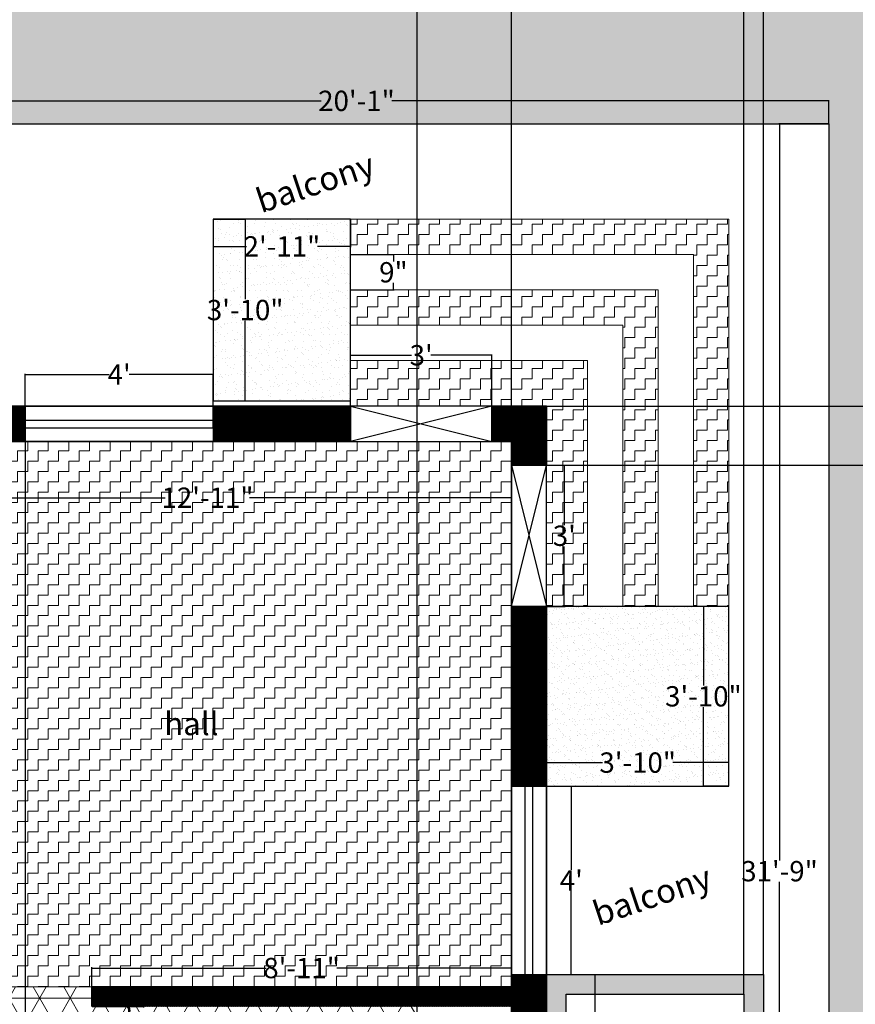
# Model space of a CAD drawing. Units: inches. Extents: x -157 to 1464, y -361 to 1077.
# Tile 6 of 9: x 463 to 676, y 268 to 519. Entities that reach past the tile are written whole.
import ezdxf

# ---------------------------------------------------------------- set-up
doc = ezdxf.new("R2010")
doc.units = ezdxf.units.IN
doc.header["$MEASUREMENT"] = 0
for name, color, linetype, lineweight in [('A-ANNO-DIMS', 2, 'Continuous', 18), ('A-AREA-IDEN', 7, 'Continuous', 18), ('A-FLOR', 7, 'Continuous', 25), ('A-FLOR-BNDY', 9, 'Continuous', 13), ('A-FLOR-PATT', 8, 'Continuous', 13), ('A-FLOR-STRS', 7, 'Continuous', 18), ('A-WALL', 7, 'Continuous', 35), ('A-WALL-PATT', 252, 'Continuous', 13), ('doors and windows', 33, 'Continuous', 25), ('L-GRND-PATT', 8, 'Continuous', 13)]:
    doc.layers.add(name, color=color, linetype=linetype, lineweight=lineweight)
doc.styles.get("Standard").update_dxf_attribs({"font": 'arial.ttf'})
doc.dimstyles.new('Annotative', dxfattribs={"dimscale": 0, "dimtxt": 5.18, "dimasz": 0.18, "dimexe": 0.18, "dimexo": 0.0625, "dimgap": 0.09, "dimtad": 0, "dimtih": 1, "dimtoh": 1, "dimdec": 0, "dimzin": 0, "dimdsep": 46, "dimlunit": 3, "dimtxsty": 'Standard', "dimcen": 0.09, "dimadec": 0, "dimazin": 0, "dimtfac": 1, "dimtdec": 0, "dimtofl": 0, "dimtmove": 0, "dimatfit": 3, "dimfxl": 1, "dimtolj": 1, "dimtzin": 0, "dimarcsym": 0})
pattern_1 = [(0, (0, 0), (2.625, 2.625), [2.625, -2.625]), (90, (2.625, 0), (-2.625, 2.625), [2.625, -2.625])]

# ---------------------------------------------------------------- blocks, each defined once
blk = doc.blocks.new('*D9')
at = {"layer": 'A-ANNO-DIMS', "color": 0, "lineweight": -2, "transparency": 16777216}
for p, q in [((463.95, 415.42), (463.95, 429.16)), ((464.13, 428.98), (485.37, 428.98)), ((511.77, 428.98), (490.53, 428.98)), ((511.95, 415.42), (511.95, 429.16))]:
    blk.add_line(p, q, dxfattribs=at)
at = {"layer": 'A-ANNO-DIMS', "color": 0, "transparency": 16777216}
for points in [[(464.13, 429.01), (464.13, 428.95), (463.95, 428.98)], [(511.77, 429.01), (511.77, 428.95), (511.95, 428.98)]]:
    blk.add_solid(points, dxfattribs=at)
at = {"layer": 'Defpoints', "color": 0, "transparency": 16777216}
for p in [(463.95, 428.98), (463.95, 415.36), (511.95, 415.36)]:
    blk.add_point(p, dxfattribs=at)
at = {"layer": 'A-ANNO-DIMS', "color": 0, "transparency": 16777216, "insert": (487.95, 428.98), "char_height": 5.18, "attachment_point": 5}
blk.add_mtext("\\A1;4'", dxfattribs=at)
blk = doc.blocks.new('*D10')
at = {"layer": 'A-ANNO-DIMS', "color": 0, "lineweight": -2, "transparency": 16777216}
for p, q in [((546.97, 420.92), (546.97, 434.07)), ((547.15, 433.89), (562.5, 433.89)), ((582.79, 433.89), (567.44, 433.89)), ((582.97, 420.92), (582.97, 434.07))]:
    blk.add_line(p, q, dxfattribs=at)
at = {"layer": 'A-ANNO-DIMS', "color": 0, "transparency": 16777216}
for points in [[(547.15, 433.92), (547.15, 433.86), (546.97, 433.89)], [(582.79, 433.92), (582.79, 433.86), (582.97, 433.89)]]:
    blk.add_solid(points, dxfattribs=at)
at = {"layer": 'Defpoints', "color": 0, "transparency": 16777216}
for p in [(582.97, 433.89), (546.97, 420.86), (582.97, 420.86)]:
    blk.add_point(p, dxfattribs=at)
at = {"layer": 'A-ANNO-DIMS', "color": 0, "transparency": 16777216, "insert": (564.97, 433.89), "char_height": 5.18, "attachment_point": 5}
blk.add_mtext("\\A1;3'", dxfattribs=at)
blk = doc.blocks.new('*D23')
at = {"layer": 'A-ANNO-DIMS', "color": 0, "lineweight": -2, "transparency": 16777216}
for p, q in [((668.9, 492.86), (656.18, 492.86)), ((656.36, 492.68), (656.36, 305.1)), ((656.36, 112.04), (656.36, 299.62)), ((668.9, 111.86), (656.18, 111.86))]:
    blk.add_line(p, q, dxfattribs=at)
at = {"layer": 'A-ANNO-DIMS', "color": 0, "transparency": 16777216}
for points in [[(656.33, 492.68), (656.39, 492.68), (656.36, 492.86)], [(656.33, 112.04), (656.39, 112.04), (656.36, 111.86)]]:
    blk.add_solid(points, dxfattribs=at)
at = {"layer": 'Defpoints', "color": 0, "transparency": 16777216}
for p in [(668.97, 492.86), (656.36, 111.86), (668.97, 111.86)]:
    blk.add_point(p, dxfattribs=at)
at = {"layer": 'A-ANNO-DIMS', "color": 0, "transparency": 16777216, "insert": (656.36, 302.36), "char_height": 5.18, "attachment_point": 5}
blk.add_mtext('\\A1;31\'-9"', dxfattribs=at)
blk = doc.blocks.new('*D24')
at = {"layer": 'A-ANNO-DIMS', "color": 0, "lineweight": -2, "transparency": 16777216}
for p, q in [((432.97, 411.8), (432.97, 397.39)), ((587.97, 411.8), (587.97, 397.39)), ((433.15, 397.57), (499.71, 397.57)), ((587.79, 397.57), (521.22, 397.57))]:
    blk.add_line(p, q, dxfattribs=at)
at = {"layer": 'A-ANNO-DIMS', "color": 0, "transparency": 16777216}
for points in [[(433.15, 397.6), (433.15, 397.54), (432.97, 397.57)], [(587.79, 397.6), (587.79, 397.54), (587.97, 397.57)]]:
    blk.add_solid(points, dxfattribs=at)
at = {"layer": 'Defpoints', "color": 0, "transparency": 16777216}
for p in [(432.97, 411.86), (587.97, 411.86), (587.97, 397.57)]:
    blk.add_point(p, dxfattribs=at)
at = {"layer": 'A-ANNO-DIMS', "color": 0, "transparency": 16777216, "insert": (510.47, 397.57), "char_height": 5.18, "attachment_point": 5}
blk.add_mtext('\\A1;12\'-11"', dxfattribs=at)
blk = doc.blocks.new('*D31')
at = {"layer": 'A-ANNO-DIMS', "color": 0, "lineweight": -2, "transparency": 16777216}
for p, q in [((511.95, 468.47), (511.95, 461.44)), ((546.97, 468.47), (546.97, 461.44)), ((512.13, 461.62), (520.43, 461.62)), ((546.79, 461.62), (538.49, 461.62))]:
    blk.add_line(p, q, dxfattribs=at)
at = {"layer": 'A-ANNO-DIMS', "color": 0, "transparency": 16777216}
for points in [[(512.13, 461.65), (512.13, 461.59), (511.95, 461.62)], [(546.79, 461.65), (546.79, 461.59), (546.97, 461.62)]]:
    blk.add_solid(points, dxfattribs=at)
at = {"layer": 'Defpoints', "color": 0, "transparency": 16777216}
for p in [(511.95, 468.53), (546.97, 468.53), (511.95, 461.62)]:
    blk.add_point(p, dxfattribs=at)
at = {"layer": 'A-ANNO-DIMS', "color": 0, "transparency": 16777216, "insert": (529.46, 461.62), "char_height": 5.18, "attachment_point": 5}
blk.add_mtext('\\A1;2\'-11"', dxfattribs=at)
blk = doc.blocks.new('*D32')
at = {"layer": 'A-ANNO-DIMS', "color": 0, "lineweight": -2, "transparency": 16777216}
for p, q in [((512.01, 468.53), (520.26, 468.53)), ((520.08, 468.35), (520.08, 448.15)), ((520.08, 422.47), (520.08, 442.68)), ((512.01, 422.29), (520.26, 422.29))]:
    blk.add_line(p, q, dxfattribs=at)
at = {"layer": 'A-ANNO-DIMS', "color": 0, "transparency": 16777216}
for points in [[(520.05, 468.35), (520.11, 468.35), (520.08, 468.53)], [(520.05, 422.47), (520.11, 422.47), (520.08, 422.29)]]:
    blk.add_solid(points, dxfattribs=at)
at = {"layer": 'Defpoints', "color": 0, "transparency": 16777216}
for p in [(511.95, 468.53), (511.95, 422.29), (520.08, 422.29)]:
    blk.add_point(p, dxfattribs=at)
at = {"layer": 'A-ANNO-DIMS', "color": 0, "transparency": 16777216, "insert": (520.08, 445.41), "char_height": 5.18, "attachment_point": 5}
blk.add_mtext('\\A1;3\'-10"', dxfattribs=at)
blk = doc.blocks.new('*D33')
at = {"layer": 'A-ANNO-DIMS', "color": 0, "lineweight": -2, "transparency": 16777216}
for p, q in [((480.97, 272.92), (480.97, 277.85)), ((481.15, 277.67), (525.48, 277.67)), ((587.79, 277.67), (543.46, 277.67)), ((587.97, 272.92), (587.97, 277.85))]:
    blk.add_line(p, q, dxfattribs=at)
at = {"layer": 'A-ANNO-DIMS', "color": 0, "transparency": 16777216}
for points in [[(481.15, 277.7), (481.15, 277.64), (480.97, 277.67)], [(587.79, 277.7), (587.79, 277.64), (587.97, 277.67)]]:
    blk.add_solid(points, dxfattribs=at)
at = {"layer": 'Defpoints', "color": 0, "transparency": 16777216}
for p in [(587.97, 277.67), (480.97, 272.86), (587.97, 272.86)]:
    blk.add_point(p, dxfattribs=at)
at = {"layer": 'A-ANNO-DIMS', "color": 0, "transparency": 16777216, "insert": (534.47, 277.67), "char_height": 5.18, "attachment_point": 5}
blk.add_mtext('\\A1;8\'-11"', dxfattribs=at)
blk = doc.blocks.new('*D38')
at = {"layer": 'A-ANNO-DIMS', "color": 0, "lineweight": -2, "transparency": 16777216}
for p, q in [((547.03, 459.53), (558.07, 459.53)), ((557.89, 459.35), (557.89, 457.77)), ((557.89, 450.71), (557.89, 452.3)), ((547.03, 450.53), (558.07, 450.53))]:
    blk.add_line(p, q, dxfattribs=at)
at = {"layer": 'A-ANNO-DIMS', "color": 0, "transparency": 16777216}
for points in [[(557.86, 459.35), (557.92, 459.35), (557.89, 459.53)], [(557.86, 450.71), (557.92, 450.71), (557.89, 450.53)]]:
    blk.add_solid(points, dxfattribs=at)
at = {"layer": 'Defpoints', "color": 0, "transparency": 16777216}
for p in [(546.97, 459.53), (557.89, 459.53), (546.97, 450.53)]:
    blk.add_point(p, dxfattribs=at)
at = {"layer": 'A-ANNO-DIMS', "color": 0, "transparency": 16777216, "insert": (557.89, 455.03), "char_height": 5.18, "attachment_point": 5}
blk.add_mtext('\\A1;9"', dxfattribs=at)
blk = doc.blocks.new('*D39')
at = {"layer": 'A-ANNO-DIMS', "color": 0, "lineweight": -2, "transparency": 16777216}
for p, q in [((597.03, 324), (603.43, 324)), ((603.25, 323.82), (603.25, 302.68)), ((603.25, 276.18), (603.25, 297.32)), ((597.03, 276), (603.43, 276))]:
    blk.add_line(p, q, dxfattribs=at)
at = {"layer": 'A-ANNO-DIMS', "color": 0, "transparency": 16777216}
for points in [[(603.22, 323.82), (603.28, 323.82), (603.25, 324)], [(603.22, 276.18), (603.28, 276.18), (603.25, 276)]]:
    blk.add_solid(points, dxfattribs=at)
at = {"layer": 'Defpoints', "color": 0, "transparency": 16777216}
for p in [(596.97, 324), (596.97, 276), (603.25, 276)]:
    blk.add_point(p, dxfattribs=at)
at = {"layer": 'A-ANNO-DIMS', "color": 0, "transparency": 16777216, "insert": (603.25, 300), "char_height": 5.18, "attachment_point": 5}
blk.add_mtext("\\A1;4'", dxfattribs=at)
blk = doc.blocks.new('*D40')
at = {"layer": 'A-ANNO-DIMS', "color": 0, "lineweight": -2, "transparency": 16777216}
for p, q in [((597.03, 405.86), (601.66, 405.86)), ((601.48, 405.68), (601.48, 390.6)), ((601.48, 370.04), (601.48, 385.12)), ((597.03, 369.86), (601.66, 369.86))]:
    blk.add_line(p, q, dxfattribs=at)
at = {"layer": 'A-ANNO-DIMS', "color": 0, "transparency": 16777216}
for points in [[(601.45, 405.68), (601.51, 405.68), (601.48, 405.86)], [(601.45, 370.04), (601.51, 370.04), (601.48, 369.86)]]:
    blk.add_solid(points, dxfattribs=at)
at = {"layer": 'Defpoints', "color": 0, "transparency": 16777216}
for p in [(596.97, 405.86), (601.48, 405.86), (596.97, 369.86)]:
    blk.add_point(p, dxfattribs=at)
at = {"layer": 'A-ANNO-DIMS', "color": 0, "transparency": 16777216, "insert": (601.48, 387.86), "char_height": 5.18, "attachment_point": 5}
blk.add_mtext("\\A1;3'", dxfattribs=at)
blk = doc.blocks.new('*D41')
at = {"layer": 'A-ANNO-DIMS', "color": 0, "lineweight": -2, "transparency": 16777216}
for p, q in [((643.35, 369.86), (636.77, 369.86)), ((636.95, 369.68), (636.95, 349.67)), ((636.95, 324.18), (636.95, 344.19)), ((643.35, 324), (636.77, 324))]:
    blk.add_line(p, q, dxfattribs=at)
at = {"layer": 'A-ANNO-DIMS', "color": 0, "transparency": 16777216}
for points in [[(636.92, 369.68), (636.98, 369.68), (636.95, 369.86)], [(636.92, 324.18), (636.98, 324.18), (636.95, 324)]]:
    blk.add_solid(points, dxfattribs=at)
at = {"layer": 'Defpoints', "color": 0, "transparency": 16777216}
for p in [(636.95, 369.86), (643.42, 369.86), (643.42, 324)]:
    blk.add_point(p, dxfattribs=at)
at = {"layer": 'A-ANNO-DIMS', "color": 0, "transparency": 16777216, "insert": (636.95, 346.93), "char_height": 5.18, "attachment_point": 5}
blk.add_mtext('\\A1;3\'-10"', dxfattribs=at)
blk = doc.blocks.new('*D42')
at = {"layer": 'A-ANNO-DIMS', "color": 0, "lineweight": -2, "transparency": 16777216}
for p, q in [((596.97, 324.06), (596.97, 330.22)), ((597.15, 330.04), (611.21, 330.04)), ((643.24, 330.04), (629.18, 330.04)), ((643.42, 324.06), (643.42, 330.22))]:
    blk.add_line(p, q, dxfattribs=at)
at = {"layer": 'A-ANNO-DIMS', "color": 0, "transparency": 16777216}
for points in [[(597.15, 330.07), (597.15, 330.01), (596.97, 330.04)], [(643.24, 330.07), (643.24, 330.01), (643.42, 330.04)]]:
    blk.add_solid(points, dxfattribs=at)
at = {"layer": 'Defpoints', "color": 0, "transparency": 16777216}
for p in [(643.42, 330.04), (596.97, 324), (643.42, 324)]:
    blk.add_point(p, dxfattribs=at)
at = {"layer": 'A-ANNO-DIMS', "color": 0, "transparency": 16777216, "insert": (620.19, 330.04), "char_height": 5.18, "attachment_point": 5}
blk.add_mtext('\\A1;3\'-10"', dxfattribs=at)
blk = doc.blocks.new('*D45')
at = {"layer": 'A-ANNO-DIMS', "color": 0, "lineweight": -2, "transparency": 16777216}
for p, q in [((596.97, 275.94), (596.97, 261.84)), ((652.25, 275.94), (652.25, 261.84)), ((597.15, 262.02), (617.53, 262.02)), ((652.07, 262.02), (631.69, 262.02))]:
    blk.add_line(p, q, dxfattribs=at)
at = {"layer": 'A-ANNO-DIMS', "color": 0, "transparency": 16777216}
for points in [[(597.15, 262.05), (597.15, 261.99), (596.97, 262.02)], [(652.07, 262.05), (652.07, 261.99), (652.25, 262.02)]]:
    blk.add_solid(points, dxfattribs=at)
at = {"layer": 'Defpoints', "color": 0, "transparency": 16777216}
for p in [(596.97, 276), (652.25, 276), (652.25, 262.02)]:
    blk.add_point(p, dxfattribs=at)
at = {"layer": 'A-ANNO-DIMS', "color": 0, "transparency": 16777216, "insert": (624.61, 262.02), "char_height": 5.18, "attachment_point": 5}
blk.add_mtext('\\A1;4\'-7"', dxfattribs=at)
blk = doc.blocks.new('*D46')
at = {"layer": 'A-ANNO-DIMS', "color": 0, "lineweight": -2, "transparency": 16777216}
for p, q in [((597.03, 276), (609.43, 276)), ((609.25, 275.82), (609.25, 244.05)), ((609.25, 206.81), (609.25, 238.58)), ((597.03, 206.63), (609.43, 206.63))]:
    blk.add_line(p, q, dxfattribs=at)
at = {"layer": 'A-ANNO-DIMS', "color": 0, "transparency": 16777216}
for points in [[(609.22, 275.82), (609.28, 275.82), (609.25, 276)], [(609.22, 206.81), (609.28, 206.81), (609.25, 206.63)]]:
    blk.add_solid(points, dxfattribs=at)
at = {"layer": 'Defpoints', "color": 0, "transparency": 16777216}
for p in [(596.97, 276), (609.25, 276), (596.97, 206.63)]:
    blk.add_point(p, dxfattribs=at)
at = {"layer": 'A-ANNO-DIMS', "color": 0, "transparency": 16777216, "insert": (609.25, 241.32), "char_height": 5.18, "attachment_point": 5}
blk.add_mtext('\\A1;5\'-9"', dxfattribs=at)
blk = doc.blocks.new('*D48')
at = {"layer": 'A-ANNO-DIMS', "color": 0, "lineweight": -2, "transparency": 16777216}
for p, q in [((481.03, 272.86), (494.39, 272.86)), ((494.21, 272.68), (494.21, 268.04)), ((481.03, 267.86), (494.39, 267.86)), ((494.21, 267.68), (494.03, 267.68)), ((494.21, 267.86), (494.21, 267.68))]:
    blk.add_line(p, q, dxfattribs=at)
at = {"layer": 'A-ANNO-DIMS', "color": 0, "transparency": 16777216}
for points in [[(494.18, 272.68), (494.24, 272.68), (494.21, 272.86)], [(494.18, 268.04), (494.24, 268.04), (494.21, 267.86)]]:
    blk.add_solid(points, dxfattribs=at)
at = {"layer": 'Defpoints', "color": 0, "transparency": 16777216}
for p in [(480.97, 272.86), (480.97, 267.86), (494.21, 267.86)]:
    blk.add_point(p, dxfattribs=at)
at = {"layer": 'A-ANNO-DIMS', "color": 0, "transparency": 16777216, "insert": (490.96, 267.68), "char_height": 5.18, "attachment_point": 5}
blk.add_mtext('\\A1;5"', dxfattribs=at)
blk = doc.blocks.new('*D57')
at = {"layer": 'A-ANNO-DIMS', "color": 0, "lineweight": -2, "transparency": 16777216}
for p, q in [((427.97, 492.92), (427.97, 498.91)), ((428.15, 498.73), (539.44, 498.73)), ((668.79, 498.73), (557.5, 498.73)), ((668.97, 492.92), (668.97, 498.91))]:
    blk.add_line(p, q, dxfattribs=at)
at = {"layer": 'A-ANNO-DIMS', "color": 0, "transparency": 16777216}
for points in [[(428.15, 498.76), (428.15, 498.7), (427.97, 498.73)], [(668.79, 498.76), (668.79, 498.7), (668.97, 498.73)]]:
    blk.add_solid(points, dxfattribs=at)
at = {"layer": 'Defpoints', "color": 0, "transparency": 16777216}
for p in [(668.97, 498.73), (427.97, 492.86), (668.97, 492.86)]:
    blk.add_point(p, dxfattribs=at)
at = {"layer": 'A-ANNO-DIMS', "color": 0, "transparency": 16777216, "insert": (548.47, 498.73), "char_height": 5.18, "attachment_point": 5}
blk.add_mtext('\\A1;20\'-1"', dxfattribs=at)
blk = doc.blocks.new('WIN-48x9')
for p, q in [((9, 48), (0, 48)), ((0, 48), (0, 0)), ((3.5, 48), (3.5, 0)), ((5.5, 48), (5.5, 0)), ((9, 48), (9, 0)), ((9, 0), (0, 0))]:
    blk.add_line(p, q)
blk = doc.blocks.new('DOOR-36x9')
for p, q in [((0, 0), (0, 9)), ((0, 9), (36, 0)), ((36, 9), (0, 0)), ((36, 9), (0, 9)), ((36, 0), (36, 9)), ((0, 0), (36, 0))]:
    blk.add_line(p, q)
blk = doc.blocks.new('*D73')
at = {"layer": 'A-ANNO-DIMS', "color": 0, "lineweight": -2, "transparency": 16777216}
for p, q in [((432.97, 411.8), (432.97, -357.73)), ((463.95, 411.8), (463.95, -357.73)), ((433.15, -357.55), (441.44, -357.55)), ((463.77, -357.55), (455.48, -357.55))]:
    blk.add_line(p, q, dxfattribs=at)
at = {"layer": 'A-ANNO-DIMS', "color": 0, "transparency": 16777216}
for points in [[(433.15, -357.52), (433.15, -357.58), (432.97, -357.55)], [(463.77, -357.52), (463.77, -357.58), (463.95, -357.55)]]:
    blk.add_solid(points, dxfattribs=at)
at = {"layer": 'Defpoints', "color": 0, "transparency": 16777216}
for p in [(432.97, 411.86), (463.95, 411.86), (463.95, -357.55)]:
    blk.add_point(p, dxfattribs=at)
at = {"layer": 'A-ANNO-DIMS', "color": 0, "transparency": 16777216, "insert": (448.46, -357.55), "char_height": 5.18, "attachment_point": 5}
blk.add_mtext('\\A1;2\'-7"', dxfattribs=at)
blk = doc.blocks.new('*D76')
at = {"layer": 'A-ANNO-DIMS', "color": 0, "lineweight": -2, "transparency": 16777216}
for p, q in [((597.03, 420.86), (1397.57, 420.86)), ((1397.39, 420.68), (1397.39, 416.1)), ((1397.39, 406.04), (1397.39, 410.62)), ((597.03, 405.86), (1397.57, 405.86))]:
    blk.add_line(p, q, dxfattribs=at)
at = {"layer": 'A-ANNO-DIMS', "color": 0, "transparency": 16777216}
for points in [[(1397.36, 420.68), (1397.42, 420.68), (1397.39, 420.86)], [(1397.36, 406.04), (1397.42, 406.04), (1397.39, 405.86)]]:
    blk.add_solid(points, dxfattribs=at)
at = {"layer": 'Defpoints', "color": 0, "transparency": 16777216}
for p in [(596.97, 420.86), (1397.39, 420.86), (596.97, 405.86)]:
    blk.add_point(p, dxfattribs=at)
at = {"layer": 'A-ANNO-DIMS', "color": 0, "transparency": 16777216, "insert": (1397.39, 413.36), "char_height": 5.18, "attachment_point": 5}
blk.add_mtext('\\A1;1\'-3"', dxfattribs=at)
blk = doc.blocks.new('*D81')
at = {"layer": 'A-ANNO-DIMS', "color": 0, "lineweight": -2, "transparency": 16777216}
for p, q in [((563.97, 144.92), (563.97, 1069.66)), ((564.15, 1069.48), (568.95, 1069.48)), ((587.79, 1069.48), (582.99, 1069.48)), ((587.97, 120.92), (587.97, 1069.66))]:
    blk.add_line(p, q, dxfattribs=at)
at = {"layer": 'A-ANNO-DIMS', "color": 0, "transparency": 16777216}
for points in [[(564.15, 1069.51), (564.15, 1069.45), (563.97, 1069.48)], [(587.79, 1069.51), (587.79, 1069.45), (587.97, 1069.48)]]:
    blk.add_solid(points, dxfattribs=at)
at = {"layer": 'Defpoints', "color": 0, "transparency": 16777216}
for p in [(587.97, 1069.48), (563.97, 144.86), (587.97, 120.86)]:
    blk.add_point(p, dxfattribs=at)
at = {"layer": 'A-ANNO-DIMS', "color": 0, "transparency": 16777216, "insert": (575.97, 1069.48), "char_height": 5.18, "attachment_point": 5}
blk.add_mtext('\\A1;2\'-0"', dxfattribs=at)
blk = doc.blocks.new('*D82')
at = {"layer": 'A-ANNO-DIMS', "color": 0, "lineweight": -2, "transparency": 16777216}
for p, q in [((647.25, 271.06), (647.25, 1069.66)), ((647.43, 1069.48), (652.07, 1069.48)), ((652.25, 276.06), (652.25, 1069.66)), ((652.25, 1069.48), (652.43, 1069.48))]:
    blk.add_line(p, q, dxfattribs=at)
at = {"layer": 'A-ANNO-DIMS', "color": 0, "transparency": 16777216}
for points in [[(647.43, 1069.51), (647.43, 1069.45), (647.25, 1069.48)], [(652.07, 1069.51), (652.07, 1069.45), (652.25, 1069.48)]]:
    blk.add_solid(points, dxfattribs=at)
at = {"layer": 'Defpoints', "color": 0, "transparency": 16777216}
for p in [(652.25, 1069.48), (652.25, 276), (647.25, 271)]:
    blk.add_point(p, dxfattribs=at)
at = {"layer": 'A-ANNO-DIMS', "color": 0, "transparency": 16777216, "insert": (659.4, 1069.48), "char_height": 5.18, "attachment_point": 5}
blk.add_mtext('\\A1;0\'-5"', dxfattribs=at)

msp = doc.modelspace()

# ---------------------------------------------------------------- hatches: boundary and pattern name
at = {"layer": 'A-FLOR-PATT'}
h = msp.add_hatch(dxfattribs=at)
h.set_pattern_fill('AR-SAND', color=256, scale=1.7)
h.paths.add_polyline_path([(546.97, 468.53), (511.95, 468.53), (511.95, 422.29), (546.97, 422.29)])
h = msp.add_hatch(dxfattribs=at)
h.set_pattern_fill('ZIGZAG', color=256, scale=21)
h.set_pattern_definition(pattern_1)
h.paths.add_polyline_path([(625.42, 450.53), (546.97, 450.53), (546.97, 441.53), (616.42, 441.53), (616.42, 369.86), (625.42, 369.86)], flags=17)
h.paths.add_polyline_path([(643.42, 468.53), (546.97, 468.53), (546.97, 459.53), (634.42, 459.53), (634.42, 369.86), (643.42, 369.86)])
h.paths.add_polyline_path([(607.42, 432.53), (546.97, 432.53), (546.97, 422.29), (546.97, 420.86), (582.97, 420.86), (596.97, 420.86), (596.97, 405.86), (596.97, 369.86), (607.42, 369.86)], flags=16)
h.paths.add_polyline_path([(560.99, 428.52), (568.98, 428.52), (568.98, 439.19), (560.99, 439.19)], flags=24)
h = msp.add_hatch(dxfattribs=at)
h.set_pattern_fill('ZIGZAG', color=256, scale=21)
h.set_pattern_definition(pattern_1)
h.paths.add_polyline_path([(587.97, 272.86), (587.97, 369.86), (587.97, 405.86), (587.97, 411.86), (582.97, 411.86), (546.97, 411.86), (432.97, 411.86), (432.97, 313.86), (427.97, 313.86), (427.97, 277.86), (432.97, 277.86), (432.97, 272.86), (480.97, 272.86)])
h.paths.add_polyline_path([(497.45, 333.85), (513.07, 333.85), (513.07, 345.88), (497.45, 345.88)], flags=24)
h = msp.add_hatch(dxfattribs=at)
h.set_pattern_fill('AR-SAND', color=256, scale=1.4)
h.paths.add_polyline_path([(643.42, 369.86), (596.97, 369.86), (596.97, 324), (643.42, 324)])
h = msp.add_hatch(color=256, dxfattribs=at)
h.dxf.hatch_style = 1
h.paths.add_polyline_path([(652.25, 276), (596.97, 276), (596.97, 206.63), (652.25, 206.63)])
h.paths.add_polyline_path([(647.25, 271), (647.25, 211.63), (601.97, 211.63), (601.97, 271)], flags=16)
h = msp.add_hatch(dxfattribs=at)
h.set_pattern_fill('NET3', color=256, scale=54)
h.paths.add_polyline_path([(563.97, 267.86), (480.97, 267.86), (480.97, 272.86), (432.97, 272.86), (432.97, 262.86), (427.97, 262.86), (427.97, 267.86), (307.97, 267.86), (307.97, 120.86), (427.97, 120.86), (427.97, 226.86), (432.97, 226.86), (432.97, 203.86), (438.97, 203.86), (468.97, 203.86), (485.97, 203.86), (485.97, 144.86), (563.97, 144.86)])
h.paths.add_polyline_path([(507.66, 186.06), (540.97, 186.06), (540.97, 198.1), (507.66, 198.1)], flags=24)
h.paths.add_polyline_path([(343.4, 209.88), (389.84, 209.88), (389.84, 221.92), (343.4, 221.92)], flags=24)
at = {"layer": 'A-WALL-PATT'}
h = msp.add_hatch(dxfattribs=at)
h.set_pattern_fill('ANSI31', color=256)
h.set_pattern_definition([(45, (213.19381, 103.60139), (-0.088388348, 0.088388348), [])])
h.paths.add_polyline_path([(307.97, 267.86), (427.97, 267.86), (427.97, 262.86), (432.97, 262.86), (432.97, 277.86), (427.97, 277.86), (427.97, 272.86), (307.97, 272.86), (307.97, 276.53), (298.97, 276.53), (298.97, 194.36), (307.97, 194.36)])
h.paths.add_polyline_path([(307.97, 411.86), (427.97, 411.86), (427.97, 313.86), (432.97, 313.86), (432.97, 411.86), (463.95, 411.86), (463.95, 420.86), (298.97, 420.86), (298.97, 324.53), (307.97, 324.53)])
h.paths.add_polyline_path([(511.95, 420.86), (511.95, 411.86), (546.97, 411.86), (546.97, 420.86)])
h.paths.add_polyline_path([(587.97, 411.86), (587.97, 405.86), (596.97, 405.86), (596.97, 420.86), (582.97, 420.86), (582.97, 411.86)])
h.paths.add_polyline_path([(587.97, 369.86), (587.97, 324), (596.97, 324), (596.97, 369.86)])
h.paths.add_polyline_path([(596.97, 276), (587.97, 276), (587.97, 272.86), (480.97, 272.86), (480.97, 267.86), (587.97, 267.86), (587.97, 206.9), (596.97, 206.9)])
h.paths.add_polyline_path([(587.97, 120.86), (485.97, 120.86), (485.97, 203.86), (468.97, 203.86), (468.97, 198.86), (480.97, 198.86), (480.97, 120.86), (465.97, 120.86), (465.97, 111.86), (596.97, 111.86), (596.97, 158.9), (587.97, 158.9)])
h.paths.add_polyline_path([(427.97, 120.86), (307.97, 120.86), (307.97, 146.36), (298.97, 146.36), (298.97, 111.86), (447.97, 111.86), (447.97, 120.86), (432.97, 120.86), (432.97, 198.86), (438.97, 198.86), (438.97, 203.86), (432.97, 203.86), (432.97, 226.86), (427.97, 226.86)])
at = {"layer": 'L-GRND-PATT'}
h = msp.add_hatch(dxfattribs=at)
h.set_pattern_fill('GRAVEL', color=256, scale=26)
h.set_pattern_definition([(228.01279, (18.72, 26), (-208, -234), [3.49794, -346.2963]), (184.96974, (16.38, 23.4), (312, 26), [6.00257, -594.25404]), (132.51045, (10.4, 22.88), (260, -286), [4.2325, -419.01685]), (267.27369, (0.26, 16.38), (26, 520), [5.4662, -541.1525]), (292.83365, (0, 10.92), (-130, 312), [5.36003, -530.6437]), (357.27369, (2.08, 5.98), (-520, 26), [5.4662, -541.1525]), (37.69424, (7.54, 5.72), (-338, -260), [7.22875, -715.64606]), (72.25533, (13.26, 10.14), (182, 572), [6.8247, -675.64436]), (121.42957, (15.34, 16.64), (-208, 338), [5.4847, -542.9859]), (175.23636, (12.48, 21.32), (286, -26), [6.26163, -306.81983]), (222.39744, (6.24, 21.84), (-312, -286), [8.09765, -801.66775]), (138.81407, (26, 16.12), (-182, 156), [2.76383, -273.61997]), (171.46923, (23.92, 17.94), (338, -52), [5.25816, -520.5593]), (225, (18.72, 18.72), (-3e-15, -26), [3.67695, -33.0926]), (203.1986, (16.9, 21.84), (130, 52), [1.9801, -196.03]), (291.8014, (15.08, 21.06), (-26, 78), [2.8003, -137.214]), (30.96376, (16.12, 18.46), (78, 52), [4.54815, -147.0566]), (161.56505, (20.02, 20.8), (52, -26), [3.28877, -78.93045]), (16.38954, (0, 21.06), (260, 78), [4.6072, -456.11397]), (70.34618, (4.42, 22.36), (-104, -286), [3.8652, -382.6526]), (293.1986, (20.02, 26), (-52, 130), [3.9602, -194.0499]), (343.61046, (21.58, 22.36), (-260, 78), [4.6072, -456.11397]), (339.44395, (0, 4.94), (-130, 52), [4.4429, -217.7012]), (294.77514, (4.16, 3.38), (-130, 286), [3.72263, -368.5407]), (66.8014, (20.28, 0), (52, 130), [3.9602, -194.0499]), (17.35402, (21.84, 3.64), (-338, -104), [4.3584, -431.481]), (69.44395, (7.54, 0), (-52, -130), [2.22144, -219.92266]), (101.30993, (18.72, 0), (-26, 104), [1.32574, -131.24877]), (165.96376, (18.46, 1.3), (78, -26), [5.36003, -101.8407]), (186.009, (13.26, 2.6), (260, 26), [4.9673, -491.762]), (303.6901, (16.12, 16.12), (-26, 52), [3.7498, -89.99456]), (353.15723, (18.2, 13), (442, -52), [6.54664, -648.11663]), (60.9454, (24.7, 12.22), (-104, -182), [2.67686, -265.00953]), (90, (26, 14.56), (-26, 26), [1.56, -24.44]), (120.25644, (12.74, 3.38), (104, -182), [3.61202, -357.5915]), (48.01279, (10.92, 6.5), (208, 234), [6.99587, -342.79835]), (0, (15.6, 11.7), (26, 26), [6.76, -19.24]), (325.30485, (22.36, 11.7), (260, -182), [4.11096, -406.98513]), (254.0546, (25.74, 9.36), (-26, -104), [3.78565, -185.4972]), (207.64598, (24.7, 5.72), (-494, -260), [6.1637, -610.20633]), (175.42608, (19.24, 2.86), (-338, 26), [6.52077, -645.5559])])
h.paths.add_polyline_path([(856.57, 645.71), (257.33, 643.42), (257.33, 70.37), (856.57, 72.66)])
h.paths.add_polyline_path([(668.97, 111.86), (596.97, 111.86), (298.97, 111.86), (298.97, 420.86), (298.97, 492.86), (427.97, 492.86), (668.97, 492.86)], flags=16)
h.paths.add_polyline_path([(842.44, 305.24), (842.44, 199.78), (692.18, 199.78), (692.18, 305.24)], flags=16)
h.paths.add_polyline_path([(596.97, 369.86), (596.97, 158.9), (587.97, 158.9), (587.97, 120.86), (485.97, 120.86), (485.97, 203.86), (468.97, 203.86), (468.97, 198.86), (480.97, 198.86), (480.97, 120.86), (465.97, 120.86), (465.97, 111.86), (447.97, 111.86), (447.97, 120.86), (432.97, 120.86), (432.97, 198.86), (438.97, 198.86), (438.97, 203.86), (432.97, 203.86), (432.97, 226.86), (427.97, 226.86), (427.97, 120.86), (307.97, 120.86), (307.97, 146.36), (298.97, 146.36), (298.97, 194.36), (307.97, 194.36), (307.97, 267.86), (427.97, 267.86), (427.97, 262.86), (432.97, 262.86), (432.97, 277.86), (427.97, 277.86), (427.97, 272.86), (307.97, 272.86), (307.97, 276.53), (298.97, 276.53), (298.97, 324.53), (307.97, 324.53), (307.97, 411.86), (427.97, 411.86), (427.97, 313.86), (432.97, 313.86), (432.97, 411.86), (463.95, 411.86), (463.95, 420.86), (334.97, 420.86), (334.97, 456.86), (427.97, 456.86), (427.97, 420.86), (546.97, 420.86), (582.97, 420.86), (596.97, 420.86), (596.97, 405.86)], flags=0)
h.paths.add_polyline_path([(596.97, 369.86), (587.97, 369.86), (587.97, 324), (596.97, 324), (596.97, 276), (587.97, 276), (587.97, 369.86), (587.97, 405.86), (587.97, 411.86), (582.97, 411.86), (546.97, 411.86), (546.97, 420.86), (564.97, 416.36), (582.97, 420.86), (582.97, 411.86), (587.97, 411.86), (587.97, 405.86), (596.97, 405.86), (592.47, 387.86)], flags=0)
h.paths.add_polyline_path([(468.97, 203.86), (468.97, 198.86), (438.97, 198.86), (438.97, 203.86)], flags=0)
h.paths.add_polyline_path([(267.35, 260.99), (288.37, 260.99), (288.37, 271.66), (267.35, 271.66)], flags=24)
h.paths.add_polyline_path([(435.51, 88.48), (460.55, 88.48), (460.55, 99.15), (435.51, 99.15)], flags=24)
h.paths.add_polyline_path([(315.69, 188.99), (336.72, 188.99), (336.72, 199.66), (315.69, 199.66)], flags=8)
h.paths.add_polyline_path([(361.73, 141.9), (373.75, 141.9), (373.75, 152.57), (361.73, 152.57)], flags=8)
h.paths.add_polyline_path([(430.38, 154.49), (447.38, 154.49), (447.38, 165.16), (430.38, 165.16)], flags=8)
h.paths.add_polyline_path([(451.09, 165.32), (468.09, 165.32), (468.09, 175.99), (451.09, 175.99)], flags=8)
h.paths.add_polyline_path([(361.73, 305.06), (373.75, 305.06), (373.75, 315.74), (361.73, 315.74)], flags=8)
h.paths.add_polyline_path([(316.13, 336.94), (337.15, 336.94), (337.15, 347.62), (316.13, 347.62)], flags=8)
h.paths.add_polyline_path([(484.07, 423.56), (492.07, 423.56), (492.07, 434.24), (484.07, 434.24)], flags=8)
h.paths.add_polyline_path([(560.99, 428.52), (568.98, 428.52), (568.98, 439.19), (560.99, 439.19)], flags=8)
h.paths.add_polyline_path([(528.49, 131.95), (545.49, 131.95), (545.49, 142.62), (528.49, 142.62)], flags=8)
h.paths.add_polyline_path([(564.53, 188.99), (585.55, 188.99), (585.55, 199.66), (564.53, 199.66)], flags=8)

# ---------------------------------------------------------------- linework, layer by layer
at = {"layer": 'A-FLOR'}
for p, q in [((427.97, 492.86), (668.97, 492.86)), ((668.97, 492.86), (668.97, 111.86))]:
    msp.add_line(p, q, dxfattribs=at)
for points in [[(511.95, 422.29), (546.97, 422.29), (546.97, 468.53), (511.95, 468.53)], [(596.97, 324), (643.42, 324), (643.42, 369.86), (596.97, 369.86)], [(596.97, 276), (652.25, 276), (652.25, 206.63), (596.97, 206.63)], [(601.97, 271), (647.25, 271), (647.25, 211.63), (601.97, 211.63)]]:
    msp.add_lwpolyline(points, close=True, dxfattribs=at)
at = {"layer": 'A-FLOR-BNDY'}
msp.add_line((480.97, 272.86), (432.97, 272.86), dxfattribs=at)
at = {"layer": 'A-FLOR-STRS'}
for p, q in [((546.97, 420.86), (546.97, 468.53)), ((643.42, 369.86), (596.97, 369.86))]:
    msp.add_line(p, q, dxfattribs=at)
for points in [[(546.97, 468.53), (643.42, 468.53), (643.42, 369.86)], [(546.97, 459.53), (634.42, 459.53), (634.42, 369.86)], [(546.97, 450.53), (625.42, 450.53), (625.42, 369.86)], [(546.97, 441.53), (616.42, 441.53), (616.42, 369.86)], [(546.97, 432.53), (607.42, 432.53), (607.42, 369.86)]]:
    msp.add_lwpolyline(points, dxfattribs=at)
at = {"layer": 'A-WALL'}
for p, q in [((298.97, 420.86), (546.97, 420.86)), ((546.97, 411.86), (546.97, 420.86)), ((582.97, 411.86), (582.97, 420.86)), ((582.97, 420.86), (596.97, 420.86)), ((596.97, 420.86), (596.97, 405.86)), ((432.97, 411.86), (546.97, 411.86)), ((582.97, 411.86), (587.97, 411.86)), ((587.97, 411.86), (587.97, 405.86)), ((587.97, 405.86), (596.97, 405.86)), ((587.97, 369.86), (596.97, 369.86)), ((587.97, 369.86), (587.97, 272.86)), ((596.97, 369.86), (596.97, 111.86)), ((480.97, 267.86), (480.97, 272.86)), ((480.97, 272.86), (587.97, 272.86))]:
    msp.add_line(p, q, dxfattribs=at)

# ---------------------------------------------------------------- block references
at = {"layer": 'doors and windows'}
for name, p, rotation in [('WIN-48x9', (511.95, 411.86), 90.00000000000011), ('DOOR-36x9', (596.97, 369.86), 89.99999999999966), ('WIN-48x9', (596.97, 324), 180)]:
    msp.add_blockref(name, p, dxfattribs=dict(at, rotation=rotation))
msp.add_blockref('DOOR-36x9', (546.97, 411.86), dxfattribs=at)

# ---------------------------------------------------------------- texts
at = {"layer": 'A-AREA-IDEN'}
for p in [(524.16, 470.05), (610.07, 288.4)]:
    msp.add_text('balcony', height=6.137, rotation=18.4487, dxfattribs=at).set_placement(p)
at = {"layer": 'A-AREA-IDEN', "insert": (499.45, 342.88), "char_height": 5.84, "attachment_point": 1}
msp.add_mtext_dynamic_manual_height_columns('hall', width=87.358, gutter_width=29.2, heights=[13.12], dxfattribs=at)

# ---------------------------------------------------------------- dimensions: what is measured, and where the dimension line sits
at = {"layer": 'A-ANNO-DIMS'}
for base, p1, p2, override, picture, middle in [((587.97, 1069.48), (563.97, 144.86), (587.97, 120.86), {"dimscale": 1, "dimdec": 1, "dimzin": 1, "dimlunit": 4, "dimfrac": 2}, '*D81', (575.97, 1069.48)), ((652.25, 1069.48), (647.25, 271), (652.25, 276), {"dimscale": 1, "dimdec": 1, "dimzin": 1, "dimlunit": 4, "dimfrac": 2}, '*D82', (659.4, 1069.48)), ((668.97, 498.73), (427.97, 492.86), (668.97, 492.86), {"dimclrd": 0, "dimclre": 0, "dimclrt": 0}, '*D57', (548.47, 498.73)), ((511.95, 461.62), (546.97, 468.53), (511.95, 468.53), {"dimclrd": 0, "dimclre": 0, "dimclrt": 0}, '*D31', (529.46, 461.62)), ((582.97, 433.89), (546.97, 420.86), (582.97, 420.86), {"dimclrd": 0, "dimclre": 0, "dimclrt": 0}, '*D10', (564.97, 433.89)), ((463.95, 428.98), (511.95, 415.36), (463.95, 415.36), {"dimclrd": 0, "dimclre": 0, "dimclrt": 0}, '*D9', (487.95, 428.98)), ((587.97, 397.57), (432.97, 411.86), (587.97, 411.86), {"dimclrd": 0, "dimclre": 0, "dimclrt": 0}, '*D24', (510.47, 397.57)), ((463.95, -357.55), (432.97, 411.86), (463.95, 411.86), {"dimscale": 1, "dimdec": 1, "dimzin": 1, "dimlunit": 4, "dimfrac": 2}, '*D73', (448.46, -357.55)), ((643.42, 330.04), (596.97, 324), (643.42, 324), {"dimclrd": 0, "dimclre": 0, "dimclrt": 0}, '*D42', (620.19, 330.04)), ((587.97, 277.67), (480.97, 272.86), (587.97, 272.86), {"dimclrd": 0, "dimclre": 0, "dimclrt": 0}, '*D33', (534.47, 277.67)), ((652.25, 262.02), (596.97, 276), (652.25, 276), {"dimclrd": 0, "dimclre": 0, "dimclrt": 0}, '*D45', (624.61, 262.02))]:
    dim = msp.add_linear_dim(base=base, p1=p1, p2=p2, dimstyle='Annotative', override=override, dxfattribs=at)
    dim.commit()
    dim.dimension.update_dxf_attribs({"geometry": picture, "text_midpoint": middle})
for base, p1, p2, override, picture, middle in [((656.36, 111.86), (668.97, 492.86), (668.97, 111.86), {"dimclrd": 0, "dimclre": 0, "dimclrt": 0}, '*D23', (656.36, 302.36)), ((520.08, 422.29), (511.95, 468.53), (511.95, 422.29), {"dimclrd": 0, "dimclre": 0, "dimclrt": 0}, '*D32', (520.08, 445.41)), ((557.89, 459.53), (546.97, 450.53), (546.97, 459.53), {"dimclrd": 0, "dimclre": 0, "dimclrt": 0}, '*D38', (557.89, 455.03)), ((1397.39, 420.86), (596.97, 405.86), (596.97, 420.86), {"dimscale": 1, "dimdec": 1, "dimzin": 1, "dimlunit": 4, "dimfrac": 2}, '*D76', (1397.39, 413.36)), ((601.48, 405.86), (596.97, 369.86), (596.97, 405.86), {"dimclrd": 0, "dimclre": 0, "dimclrt": 0}, '*D40', (601.48, 387.86)), ((636.95, 369.86), (643.42, 324), (643.42, 369.86), {"dimclrd": 0, "dimclre": 0, "dimclrt": 0}, '*D41', (636.95, 346.93)), ((603.25, 276), (596.97, 324), (596.97, 276), {"dimclrd": 0, "dimclre": 0, "dimclrt": 0}, '*D39', (603.25, 300)), ((609.25, 276), (596.97, 206.63), (596.97, 276), {"dimclrd": 0, "dimclre": 0, "dimclrt": 0}, '*D46', (609.25, 241.32)), ((494.21, 267.86), (480.97, 272.86), (480.97, 267.86), {"dimclrd": 0, "dimclre": 0, "dimclrt": 0}, '*D48', (490.96, 267.68))]:
    dim = msp.add_linear_dim(base=base, p1=p1, p2=p2, angle=90, dimstyle='Annotative', override=override, dxfattribs=at)
    dim.commit()
    dim.dimension.update_dxf_attribs({"geometry": picture, "text_midpoint": middle})

doc.saveas('drawing.dxf')
